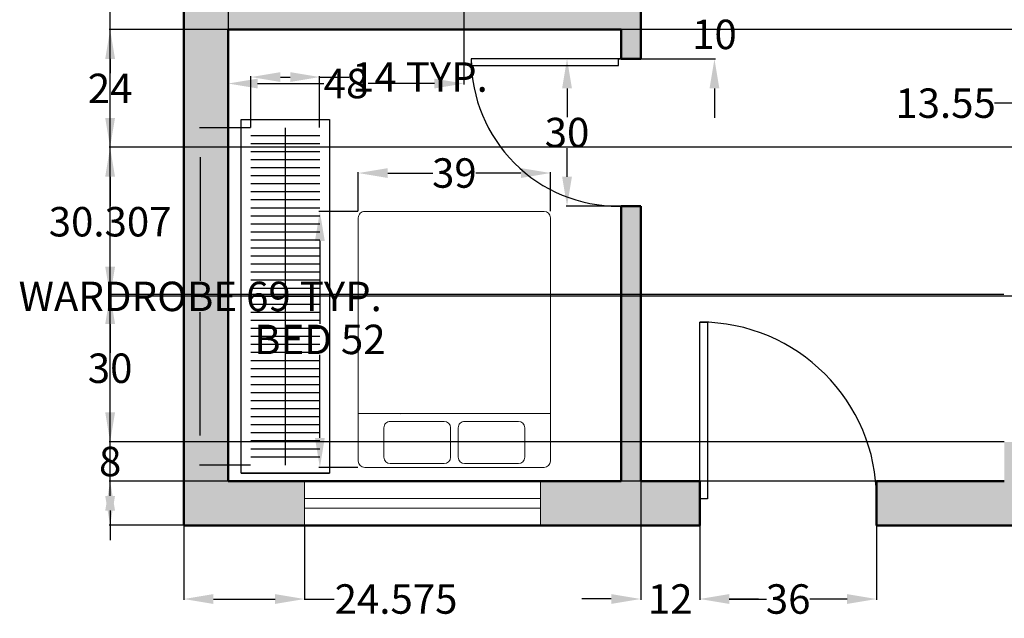
# Model space of a CAD drawing. Units: inches. Extents: x -11 to 341, y -300 to 41.
# Tile 1 of 5: x -9 to 192, y -300 to -178. Entities that reach past the tile are written whole.
import ezdxf

# ---------------------------------------------------------------- set-up
doc = ezdxf.new("R2010")
doc.units = ezdxf.units.IN
doc.header["$MEASUREMENT"] = 0
for name, color, linetype, lineweight in [('A-ANNO-DIMS', 2, 'Continuous', 18), ('A-DOOR', 3, 'Continuous', 25), ('A-FLOR-CASE', 8, 'Continuous', 25), ('A-FURN', 8, 'Continuous', 18), ('A-GLAZ', 4, 'Continuous', 18), ('A-WALL', 7, 'Continuous', 50), ('A-WALL-PATT', 251, 'Continuous', 13)]:
    doc.layers.add(name, color=color, linetype=linetype, lineweight=lineweight)
doc.styles.get("Standard").update_dxf_attribs({"font": 'arial.ttf'})
doc.dimstyles.get("Standard").update_dxf_attribs({"dimtxt": 6, "dimasz": 6, "dimexe": 0.18, "dimexo": 0.0625, "dimgap": 0.09, "dimtad": 0, "dimtih": 1, "dimtoh": 1, "dimdec": 0, "dimzin": 0, "dimdsep": 46, "dimlunit": 4, "dimtxsty": 'Standard', "dimcen": 0.09, "dimadec": 0, "dimazin": 0, "dimtfac": 1, "dimtdec": 0, "dimtofl": 0, "dimtmove": 0, "dimatfit": 3, "dimfxl": 1, "dimtolj": 1, "dimtzin": 0, "dimarcsym": 0})

# ---------------------------------------------------------------- blocks, each defined once
blk = doc.blocks.new('*U13')
for p, q in [((0, 0), (0, 6)), ((40, 0), (40, 6))]:
    blk.add_line(p, q)
blk.add_lwpolyline([(0, 0), (0, -40), (1.75, -40), (1.75, 0)], close=True)
blk.add_arc((0, 0), 40, 270, 0)
blk = doc.blocks.new('*U12')
for p, q in [((0, 0), (0, -6)), ((40, 0), (40, -6))]:
    blk.add_line(p, q)
blk.add_lwpolyline([(0, 0), (0, 40), (1.75, 40), (1.75, 0)], close=True)
blk.add_arc((0, 0), 40, 0, 90)
blk = doc.blocks.new('Bed - Queen')
for p, q in [((2, 0), (57.99999, 0)), ((0, -78.00003), (0, -2)), ((9.99999, -1.2), (26.79998, -1.2)), ((33.19999, -1.2), (49.99999, -1.2)), ((59.99999, -2), (59.99999, -78.00003)), ((7.99999, -12.4), (7.99999, -3.2)), ((28.79998, -3.2), (28.79998, -12.4)), ((31.19999, -12.4), (31.19999, -3.2)), ((51.99999, -3.2), (51.99999, -12.4)), ((9.99999, -14.4), (26.79998, -14.4)), ((33.19999, -14.4), (49.99999, -14.4)), ((59.99999, -16.8), (0, -16.8)), ((46.8, -16.4), (46.79936, -16.4)), ((57.99999, -80.00003), (2, -80.00003))]:
    blk.add_line(p, q)
for centre, start, end in [((2, -2), 90, 180), ((57.99999, -2), 0, 90), ((9.99999, -3.2), 90, 180), ((26.79998, -3.2), 0, 90), ((33.19999, -3.2), 90, 180), ((49.99999, -3.2), 0, 90), ((9.99999, -12.4), 180, 270), ((26.79998, -12.4), 270, 0), ((33.19999, -12.4), 180, 270), ((49.99999, -12.4), 270, 0), ((2, -78.00003), 180, 270), ((57.99999, -78.00003), 270, 0)]:
    blk.add_arc(centre, 2, start, end)
blk = doc.blocks.new('WIN-48IN')
for p, q in [((0, 0), (0, 9)), ((48, 9), (48, 0)), ((0, 5.5), (48, 5.5)), ((0, 3.5), (48, 3.5))]:
    blk.add_line(p, q)
blk = doc.blocks.new('WARDROBE-HANGING-RAIL')
for p, q in [((7, 68.73), (7, 0)), ((14, 67.09), (0, 67.09)), ((14, 65.45), (0, 65.45)), ((14, 63.82), (0, 63.82)), ((14, 62.18), (0, 62.18)), ((14, 60.55), (0, 60.55)), ((14, 58.91), (0, 58.91)), ((14, 57.27), (0, 57.27)), ((14, 55.64), (0, 55.64)), ((14, 54), (0, 54)), ((14, 52.36), (0, 52.36)), ((14, 50.73), (0, 50.73)), ((14, 49.09), (0, 49.09)), ((14, 47.45), (0, 47.45)), ((14, 45.82), (0, 45.82)), ((14, 44.18), (0, 44.18)), ((14, 42.55), (0, 42.55)), ((14, 40.91), (0, 40.91)), ((14, 39.27), (0, 39.27)), ((14, 37.64), (0, 37.64)), ((14, 36), (0, 36)), ((14, 34.36), (0, 34.36)), ((14, 32.73), (0, 32.73)), ((14, 31.09), (0, 31.09)), ((14, 29.45), (0, 29.45)), ((14, 27.82), (0, 27.82)), ((14, 26.18), (0, 26.18)), ((14, 24.55), (0, 24.55)), ((14, 22.91), (0, 22.91)), ((14, 21.27), (0, 21.27)), ((14, 19.64), (0, 19.64)), ((14, 18), (0, 18)), ((14, 16.36), (0, 16.36)), ((14, 14.73), (0, 14.73)), ((14, 13.09), (0, 13.09)), ((14, 11.45), (0, 11.45)), ((14, 9.82), (0, 9.82)), ((14, 8.18), (0, 8.18)), ((14, 6.55), (0, 6.55)), ((14, 4.91), (0, 4.91)), ((14, 3.27), (0, 3.27)), ((14, 1.64), (0, 1.64))]:
    blk.add_line(p, q)
blk = doc.blocks.new('*D23')
at = {"layer": 'A-ANNO-DIMS', "color": 0, "lineweight": -2, "transparency": 16777216}
for p, q in [((60.01, -216.66), (52.07, -216.66)), ((52.25, -222.66), (52.25, -239.58)), ((52.25, -262.81), (52.25, -245.89)), ((60.01, -268.81), (52.07, -268.81))]:
    blk.add_line(p, q, dxfattribs=at)
at = {"layer": 'A-ANNO-DIMS', "color": 0, "transparency": 16777216}
for points in [[(51.25, -222.66), (53.25, -222.66), (52.25, -216.66)], [(51.25, -262.81), (53.25, -262.81), (52.25, -268.81)]]:
    blk.add_solid(points, dxfattribs=at)
at = {"layer": 'Defpoints', "color": 0, "transparency": 16777216}
for p in [(60.08, -216.66), (52.25, -268.81), (60.08, -268.81)]:
    blk.add_point(p, dxfattribs=at)
at = {"layer": 'A-ANNO-DIMS', "color": 0, "transparency": 16777216, "insert": (52.25, -242.73), "char_height": 6, "attachment_point": 5}
blk.add_mtext('\\A1;BED 52', dxfattribs=at)
blk = doc.blocks.new('*D24')
at = {"layer": 'A-ANNO-DIMS', "color": 0, "lineweight": -2, "transparency": 16777216}
for p, q in [((60.08, -216.6), (60.08, -208.66)), ((66.08, -208.84), (75.24, -208.84)), ((93.18, -208.84), (84.02, -208.84)), ((99.18, -216.6), (99.18, -208.66))]:
    blk.add_line(p, q, dxfattribs=at)
at = {"layer": 'A-ANNO-DIMS', "color": 0, "transparency": 16777216}
for points in [[(66.08, -207.84), (66.08, -209.84), (60.08, -208.84)], [(93.18, -207.84), (93.18, -209.84), (99.18, -208.84)]]:
    blk.add_solid(points, dxfattribs=at)
at = {"layer": 'Defpoints', "color": 0, "transparency": 16777216}
for p in [(60.08, -208.84), (60.08, -216.66), (99.18, -216.66)]:
    blk.add_point(p, dxfattribs=at)
at = {"layer": 'A-ANNO-DIMS', "color": 0, "transparency": 16777216, "insert": (79.63, -208.84), "char_height": 6, "attachment_point": 5}
blk.add_mtext('\\A1;39', dxfattribs=at)
blk = doc.blocks.new('*D27')
at = {"layer": 'A-ANNO-DIMS', "color": 0, "lineweight": -2, "transparency": 16777216}
for p, q in [((38.15, -199.6), (27.72, -199.6)), ((27.9, -205.6), (27.9, -230.77)), ((27.9, -262.33), (27.9, -237.16)), ((38.15, -268.33), (27.72, -268.33))]:
    blk.add_line(p, q, dxfattribs=at)
at = {"layer": 'A-ANNO-DIMS', "color": 0, "transparency": 16777216}
for points in [[(26.9, -205.6), (28.9, -205.6), (27.9, -199.6)], [(26.9, -262.33), (28.9, -262.33), (27.9, -268.33)]]:
    blk.add_solid(points, dxfattribs=at)
at = {"layer": 'Defpoints', "color": 0, "transparency": 16777216}
for p in [(27.9, -199.6), (38.21, -199.6), (38.21, -268.33)]:
    blk.add_point(p, dxfattribs=at)
at = {"layer": 'A-ANNO-DIMS', "color": 0, "transparency": 16777216, "insert": (27.9, -233.97), "char_height": 6, "attachment_point": 5}
blk.add_mtext('\\A1;WARDROBE 69 TYP.', dxfattribs=at)
blk = doc.blocks.new('*D28')
at = {"layer": 'A-ANNO-DIMS', "color": 0, "lineweight": -2, "transparency": 16777216}
for p, q in [((38.21, -199.54), (38.21, -189.11)), ((44.21, -189.29), (46.21, -189.29)), ((52.21, -199.54), (52.21, -189.11)), ((52.21, -189.29), (58.21, -189.29))]:
    blk.add_line(p, q, dxfattribs=at)
at = {"layer": 'A-ANNO-DIMS', "color": 0, "transparency": 16777216}
for points in [[(44.21, -188.29), (44.21, -190.29), (38.21, -189.29)], [(46.21, -188.29), (46.21, -190.29), (52.21, -189.29)]]:
    blk.add_solid(points, dxfattribs=at)
at = {"layer": 'Defpoints', "color": 0, "transparency": 16777216}
for p in [(52.21, -189.29), (38.21, -199.6), (52.21, -199.6)]:
    blk.add_point(p, dxfattribs=at)
at = {"layer": 'A-ANNO-DIMS', "color": 0, "transparency": 16777216, "insert": (72.62, -189.29), "char_height": 6, "attachment_point": 5}
blk.add_mtext('\\A1;14 TYP.', dxfattribs=at)
blk = doc.blocks.new('*D46')
at = {"layer": 'A-ANNO-DIMS', "color": 0, "lineweight": -2, "transparency": 16777216}
for p, q in [((24.5, 19.4), (9.38, 19.4)), ((9.56, 13.4), (9.56, -127.45)), ((9.56, -274.6), (9.56, -133.76)), ((24.5, -280.6), (9.38, -280.6))]:
    blk.add_line(p, q, dxfattribs=at)
at = {"layer": 'A-ANNO-DIMS', "color": 0, "transparency": 16777216}
for points in [[(8.56, 13.4), (10.56, 13.4), (9.56, 19.4)], [(8.56, -274.6), (10.56, -274.6), (9.56, -280.6)]]:
    blk.add_solid(points, dxfattribs=at)
at = {"layer": 'Defpoints', "color": 0, "transparency": 16777216}
for p in [(9.56, 19.4), (24.57, 19.4), (24.57, -280.6)]:
    blk.add_point(p, dxfattribs=at)
at = {"layer": 'A-ANNO-DIMS', "color": 0, "transparency": 16777216, "insert": (9.56, -130.6), "char_height": 6, "attachment_point": 5}
blk.add_mtext('\\A1;300', dxfattribs=at)
blk = doc.blocks.new('*D50')
at = {"layer": 'A-ANNO-DIMS', "color": 0, "lineweight": -2, "transparency": 16777216}
for p, q in [((24.57, -280.67), (24.57, -295.79)), ((49.14, -280.67), (49.14, -295.79)), ((30.57, -295.61), (43.14, -295.61)), ((49.14, -295.61), (55.14, -295.61))]:
    blk.add_line(p, q, dxfattribs=at)
at = {"layer": 'A-ANNO-DIMS', "color": 0, "transparency": 16777216}
for points in [[(30.57, -294.61), (30.57, -296.61), (24.57, -295.61)], [(43.14, -294.61), (43.14, -296.61), (49.14, -295.61)]]:
    blk.add_solid(points, dxfattribs=at)
at = {"layer": 'Defpoints', "color": 0, "transparency": 16777216}
for p in [(24.57, -280.6), (49.14, -280.6), (49.14, -295.61)]:
    blk.add_point(p, dxfattribs=at)
at = {"layer": 'A-ANNO-DIMS', "color": 0, "transparency": 16777216, "insert": (67.76, -295.61), "char_height": 6, "attachment_point": 5}
blk.add_mtext('\\A1;24.575', dxfattribs=at)
blk = doc.blocks.new('*D51')
at = {"layer": 'A-ANNO-DIMS', "color": 0, "lineweight": -2, "transparency": 16777216}
for p, q in [((117.565121, -271.665765), (117.565121, -295.785265)), ((129.565121, -271.665765), (129.565121, -295.785265)), ((111.565121, -295.605265), (105.565121, -295.605265)), ((135.565121, -295.605265), (141.565121, -295.605265))]:
    blk.add_line(p, q, dxfattribs=at)
at = {"layer": 'A-ANNO-DIMS', "color": 0, "transparency": 16777216}
for points in [[(111.565121, -294.605265), (111.565121, -296.605265), (117.565121, -295.605265)], [(135.565121, -294.605265), (135.565121, -296.605265), (129.565121, -295.605265)]]:
    blk.add_solid(points, dxfattribs=at)
at = {"layer": 'Defpoints', "color": 0, "transparency": 16777216}
for p in [(117.565121, -271.603265), (129.565121, -271.603265), (129.565121, -295.605265)]:
    blk.add_point(p, dxfattribs=at)
at = {"layer": 'A-ANNO-DIMS', "color": 0, "transparency": 16777216, "insert": (123.565121, -295.605265), "char_height": 6, "attachment_point": 5}
blk.add_mtext('\\A1;12', dxfattribs=at)
blk = doc.blocks.new('*D52')
at = {"layer": 'A-ANNO-DIMS', "color": 0, "lineweight": -2, "transparency": 16777216}
for p, q in [((129.57, -280.67), (129.57, -295.79)), ((165.57, -280.67), (165.57, -295.79)), ((135.57, -295.61), (143.18, -295.61)), ((159.57, -295.61), (151.95, -295.61))]:
    blk.add_line(p, q, dxfattribs=at)
at = {"layer": 'A-ANNO-DIMS', "color": 0, "transparency": 16777216}
for points in [[(135.57, -294.61), (135.57, -296.61), (129.57, -295.61)], [(159.57, -294.61), (159.57, -296.61), (165.57, -295.61)]]:
    blk.add_solid(points, dxfattribs=at)
at = {"layer": 'Defpoints', "color": 0, "transparency": 16777216}
for p in [(129.57, -280.6), (165.57, -280.6), (165.57, -295.61)]:
    blk.add_point(p, dxfattribs=at)
at = {"layer": 'A-ANNO-DIMS', "color": 0, "transparency": 16777216, "insert": (147.57, -295.61), "char_height": 6, "attachment_point": 5}
blk.add_mtext('\\A1;36', dxfattribs=at)
blk = doc.blocks.new('*D61')
at = {"layer": 'A-ANNO-DIMS', "color": 0, "lineweight": -2, "transparency": 16777216}
for p, q in [((33.57, -175.67), (33.57, -190.79)), ((81.57, -175.67), (81.57, -190.79)), ((39.57, -190.61), (53.05, -190.61)), ((75.57, -190.61), (62.08, -190.61))]:
    blk.add_line(p, q, dxfattribs=at)
at = {"layer": 'A-ANNO-DIMS', "color": 0, "transparency": 16777216}
for points in [[(39.57, -189.61), (39.57, -191.61), (33.57, -190.61)], [(75.57, -189.61), (75.57, -191.61), (81.57, -190.61)]]:
    blk.add_solid(points, dxfattribs=at)
at = {"layer": 'Defpoints', "color": 0, "transparency": 16777216}
for p in [(33.57, -175.6), (81.57, -175.6), (33.57, -190.61)]:
    blk.add_point(p, dxfattribs=at)
at = {"layer": 'A-ANNO-DIMS', "color": 0, "transparency": 16777216, "insert": (57.57, -190.61), "char_height": 6, "attachment_point": 5}
blk.add_mtext('\\A1;48', dxfattribs=at)
blk = doc.blocks.new('*D70')
at = {"layer": 'A-ANNO-DIMS', "color": 0, "lineweight": -2, "transparency": 16777216}
for p, q in [((132.567121, -169.603265), (132.567121, -163.603265)), ((117.627621, -175.603265), (132.747121, -175.603265)), ((117.627621, -185.603265), (132.747121, -185.603265)), ((132.567121, -191.603265), (132.567121, -197.603265))]:
    blk.add_line(p, q, dxfattribs=at)
at = {"layer": 'A-ANNO-DIMS', "color": 0, "transparency": 16777216}
for points in [[(131.567121, -169.603265), (133.567121, -169.603265), (132.567121, -175.603265)], [(131.567121, -191.603265), (133.567121, -191.603265), (132.567121, -185.603265)]]:
    blk.add_solid(points, dxfattribs=at)
at = {"layer": 'Defpoints', "color": 0, "transparency": 16777216}
for p in [(117.565121, -175.603265), (117.565121, -185.603265), (132.567121, -185.603265)]:
    blk.add_point(p, dxfattribs=at)
at = {"layer": 'A-ANNO-DIMS', "color": 0, "transparency": 16777216, "insert": (132.567121, -180.603265), "char_height": 6, "attachment_point": 5}
blk.add_mtext('\\A1;10', dxfattribs=at)
blk = doc.blocks.new('*D71')
at = {"layer": 'A-ANNO-DIMS', "color": 0, "lineweight": -2, "transparency": 16777216}
for p, q in [((117.5, -185.6), (102.38, -185.6)), ((102.56, -191.6), (102.56, -197.45)), ((102.56, -209.6), (102.56, -203.76)), ((117.5, -215.6), (102.38, -215.6))]:
    blk.add_line(p, q, dxfattribs=at)
at = {"layer": 'A-ANNO-DIMS', "color": 0, "transparency": 16777216}
for points in [[(101.56, -191.6), (103.56, -191.6), (102.56, -185.6)], [(101.56, -209.6), (103.56, -209.6), (102.56, -215.6)]]:
    blk.add_solid(points, dxfattribs=at)
at = {"layer": 'Defpoints', "color": 0, "transparency": 16777216}
for p in [(102.56, -185.6), (117.57, -185.6), (117.57, -215.6)]:
    blk.add_point(p, dxfattribs=at)
at = {"layer": 'A-ANNO-DIMS', "color": 0, "transparency": 16777216, "insert": (102.56, -200.6), "char_height": 6, "attachment_point": 5}
blk.add_mtext('\\A1;30', dxfattribs=at)
blk = doc.blocks.new('*D72')
at = {"layer": 'A-ANNO-DIMS', "color": 0, "lineweight": -2, "transparency": 16777216}
for p, q in [((9.563121, -257.603265), (9.563121, -251.603265)), ((191.502621, -263.603265), (9.383121, -263.603265)), ((191.502621, -271.603265), (9.383121, -271.603265)), ((9.563121, -277.603265), (9.563121, -283.603265))]:
    blk.add_line(p, q, dxfattribs=at)
at = {"layer": 'A-ANNO-DIMS', "color": 0, "transparency": 16777216}
for points in [[(8.563121, -257.603265), (10.563121, -257.603265), (9.563121, -263.603265)], [(8.563121, -277.603265), (10.563121, -277.603265), (9.563121, -271.603265)]]:
    blk.add_solid(points, dxfattribs=at)
at = {"layer": 'Defpoints', "color": 0, "transparency": 16777216}
for p in [(191.565121, -263.603265), (9.563121, -271.603265), (191.565121, -271.603265)]:
    blk.add_point(p, dxfattribs=at)
at = {"layer": 'A-ANNO-DIMS', "color": 0, "transparency": 16777216, "insert": (9.563121, -267.603265), "char_height": 6, "attachment_point": 5}
blk.add_mtext('\\A1;8', dxfattribs=at)
blk = doc.blocks.new('*D73')
at = {"layer": 'A-ANNO-DIMS', "color": 0, "lineweight": -2, "transparency": 16777216}
for p, q in [((191.5, -233.6), (9.38, -233.6)), ((9.56, -239.6), (9.56, -245.45)), ((9.56, -257.6), (9.56, -251.76)), ((191.5, -263.6), (9.38, -263.6))]:
    blk.add_line(p, q, dxfattribs=at)
at = {"layer": 'A-ANNO-DIMS', "color": 0, "transparency": 16777216}
for points in [[(8.56, -239.6), (10.56, -239.6), (9.56, -233.6)], [(8.56, -257.6), (10.56, -257.6), (9.56, -263.6)]]:
    blk.add_solid(points, dxfattribs=at)
at = {"layer": 'Defpoints', "color": 0, "transparency": 16777216}
for p in [(9.56, -233.6), (191.57, -233.6), (191.57, -263.6)]:
    blk.add_point(p, dxfattribs=at)
at = {"layer": 'A-ANNO-DIMS', "color": 0, "transparency": 16777216, "insert": (9.56, -248.6), "char_height": 6, "attachment_point": 5}
blk.add_mtext('\\A1;30', dxfattribs=at)
blk = doc.blocks.new('*D74')
at = {"layer": 'A-ANNO-DIMS', "color": 0, "lineweight": -2, "transparency": 16777216}
for p, q in [((209.05, -179.6), (9.38, -179.6)), ((9.56, -185.6), (9.56, -188.5)), ((9.56, -197.6), (9.56, -194.71)), ((209.05, -203.6), (9.38, -203.6))]:
    blk.add_line(p, q, dxfattribs=at)
at = {"layer": 'A-ANNO-DIMS', "color": 0, "transparency": 16777216}
for points in [[(8.56, -185.6), (10.56, -185.6), (9.56, -179.6)], [(8.56, -197.6), (10.56, -197.6), (9.56, -203.6)]]:
    blk.add_solid(points, dxfattribs=at)
at = {"layer": 'Defpoints', "color": 0, "transparency": 16777216}
for p in [(209.11, -179.6), (9.56, -203.6), (209.11, -203.6)]:
    blk.add_point(p, dxfattribs=at)
at = {"layer": 'A-ANNO-DIMS', "color": 0, "transparency": 16777216, "insert": (9.56, -191.6), "char_height": 6, "attachment_point": 5}
blk.add_mtext('\\A1;24', dxfattribs=at)
blk = doc.blocks.new('*D75')
at = {"layer": 'A-ANNO-DIMS', "color": 0, "lineweight": -2, "transparency": 16777216}
for p, q in [((195.57, -179.67), (195.57, -194.79)), ((209.11, -179.67), (209.11, -194.79)), ((195.57, -194.61), (189.57, -194.61)), ((203.11, -194.61), (201.57, -194.61))]:
    blk.add_line(p, q, dxfattribs=at)
at = {"layer": 'A-ANNO-DIMS', "color": 0, "transparency": 16777216}
for points in [[(201.57, -193.61), (201.57, -195.61), (195.57, -194.61)], [(203.11, -193.61), (203.11, -195.61), (209.11, -194.61)]]:
    blk.add_solid(points, dxfattribs=at)
at = {"layer": 'Defpoints', "color": 0, "transparency": 16777216}
for p in [(195.57, -179.6), (209.11, -179.6), (195.57, -194.61)]:
    blk.add_point(p, dxfattribs=at)
at = {"layer": 'A-ANNO-DIMS', "color": 0, "transparency": 16777216, "insert": (179.61, -194.61), "char_height": 6, "attachment_point": 5}
blk.add_mtext('\\A1;13.55', dxfattribs=at)
blk = doc.blocks.new('*D76')
at = {"layer": 'A-ANNO-DIMS', "color": 0, "lineweight": -2, "transparency": 16777216}
for p, q in [((255.5, -203.6), (9.38, -203.6)), ((9.56, -209.6), (9.56, -215.6)), ((9.56, -227.91), (9.56, -221.91)), ((255.5, -233.91), (9.38, -233.91))]:
    blk.add_line(p, q, dxfattribs=at)
at = {"layer": 'A-ANNO-DIMS', "color": 0, "transparency": 16777216}
for points in [[(8.56, -209.6), (10.56, -209.6), (9.56, -203.6)], [(8.56, -227.91), (10.56, -227.91), (9.56, -233.91)]]:
    blk.add_solid(points, dxfattribs=at)
at = {"layer": 'Defpoints', "color": 0, "transparency": 16777216}
for p in [(9.56, -203.6), (255.57, -203.6), (255.57, -233.91)]:
    blk.add_point(p, dxfattribs=at)
at = {"layer": 'A-ANNO-DIMS', "color": 0, "transparency": 16777216, "insert": (9.56, -218.76), "char_height": 6, "attachment_point": 5}
blk.add_mtext('\\A1;30.307', dxfattribs=at)

msp = doc.modelspace()

# ---------------------------------------------------------------- hatches: boundary and pattern name
at = {"layer": 'A-WALL-PATT'}
h = msp.add_hatch(color=256, dxfattribs=at)
h.dxf.hatch_style = 1
h.paths.add_polyline_path([(24.5651, -280.6033), (49.1398, -280.6033), (49.1398, -271.6033), (33.5651, -271.6033), (33.5651, -179.6033), (113.5651, -179.6033), (113.5651, -185.6033), (117.5651, -185.6033), (117.5651, -175.6033), (85.5651, -175.6033), (85.5651, -127.6033), (81.5651, -127.6033), (81.5651, -175.6033), (33.5651, -175.6033), (33.5651, -138.096), (24.5651, -138.096)])
h = msp.add_hatch(color=256, dxfattribs=at)
h.dxf.hatch_style = 1
h.paths.add_polyline_path([(129.5651, -271.6033), (117.5651, -271.6033), (117.5651, -215.6033), (113.5651, -215.6033), (113.5651, -271.6033), (97.1398, -271.6033), (97.1398, -280.6033), (129.5651, -280.6033), (129.5651, -275.2033)])
h = msp.add_hatch(color=256, dxfattribs=at)
h.dxf.hatch_style = 1
h.paths.add_polyline_path([(215.5868, -280.6033), (215.5868, -271.6033), (195.5651, -271.6033), (195.5651, -263.6033), (191.5651, -263.6033), (191.5651, -271.6033), (165.5651, -271.6033), (165.5651, -280.6033)])

# ---------------------------------------------------------------- linework, layer by layer
at = {"layer": 'A-FLOR-CASE'}
msp.add_lwpolyline([(36.2111, -269.9669), (36.2111, -197.9669), (54.2111, -197.9669), (54.2111, -269.9669), (36.2111, -269.9669), (54.2111, -269.9669)], dxfattribs=at)
at = {"layer": 'A-WALL'}
for p, q in [((117.5651, -185.6033), (117.5651, -175.6033)), ((33.5651, -271.6033), (33.5651, -179.6033)), ((113.5651, -179.6033), (33.5651, -179.6033)), ((113.5651, -185.6033), (113.5651, -179.6033)), ((113.5651, -185.6033), (117.5651, -185.6033)), ((113.5651, -271.6033), (113.5651, -215.6033)), ((113.5651, -215.6033), (117.5651, -215.6033)), ((117.5651, -271.6033), (117.5651, -215.6033)), ((113.5651, -271.6033), (33.5651, -271.6033)), ((129.5651, -271.6033), (117.5651, -271.6033)), ((129.5651, -271.6033), (129.5651, -280.6033)), ((191.5651, -271.6033), (165.5651, -271.6033)), ((165.5651, -271.6033), (165.5651, -280.6033))]:
    msp.add_line(p, q, dxfattribs=at)
msp.add_lwpolyline([(129.5651, -280.6033), (24.5651, -280.6033), (24.5651, 19.3967), (288.5651, 19.3967), (288.5651, -280.6033), (165.5651, -280.6033)], dxfattribs=at)

# ---------------------------------------------------------------- block references
at = {"layer": 'A-DOOR', "xscale": 0.75, "yscale": 0.75, "zscale": 0.75, "rotation": 270}
msp.add_blockref('*U13', (113.0651, -185.6033), dxfattribs=at)
at = {"layer": 'A-DOOR', "xscale": 0.9, "yscale": 0.9, "zscale": 0.9}
msp.add_blockref('*U12', (129.5651, -275.2033), dxfattribs=at)
at = {"layer": 'A-FLOR-CASE'}
msp.add_blockref('WARDROBE-HANGING-RAIL', (38.2115, -268.3304), dxfattribs=at)
at = {"layer": 'A-FURN', "xscale": 0.6518282349868454, "yscale": 0.6518282349868454, "zscale": 0.6518282349868454, "rotation": 180}
msp.add_blockref('Bed - Queen', (99.1848, -268.8057), dxfattribs=at)
at = {"layer": 'A-GLAZ'}
msp.add_blockref('WIN-48IN', (49.1397, -280.603), dxfattribs=at)

# ---------------------------------------------------------------- dimensions: what is measured, and where the dimension line sits
at = {"layer": 'A-ANNO-DIMS'}
for base, p1, p2, angle, override, picture, middle in [((9.5631, 19.3967), (24.5651, -280.6033), (24.5651, 19.3967), 90, {"dimdec": 0, "dimlfac": 1, "dimrnd": 0, "dimzin": 0, "dimdsep": 46, "dimlunit": 2}, '*D46', (9.5631, -130.6033)), ((132.5671, -185.6033), (117.5651, -175.6033), (117.5651, -185.6033), 270, {"dimdec": 0, "dimlfac": 1, "dimrnd": 0, "dimzin": 0, "dimdsep": 46, "dimlunit": 2}, '*D70', (132.5671, -180.6033)), ((33.5651, -190.6053), (81.5651, -175.6033), (33.5651, -175.6033), 180, {"dimdec": 0, "dimlfac": 1, "dimrnd": 0, "dimzin": 0, "dimdsep": 46, "dimlunit": 2}, '*D61', (57.5651, -190.6053)), ((9.5631, -203.6033), (209.1143, -179.6033), (209.1143, -203.6033), 90, {"dimdec": 0, "dimlfac": 1, "dimrnd": 0, "dimzin": 0, "dimdsep": 46, "dimlunit": 2}, '*D74', (9.5631, -191.6033)), ((195.5651, -194.6053), (209.1143, -179.6033), (195.5651, -179.6033), 180, {"dimdec": 2, "dimlfac": 1, "dimrnd": 0, "dimzin": 0, "dimdsep": 46, "dimlunit": 2}, '*D75', (179.6115, -194.6053)), ((102.5631, -185.6033), (117.5651, -215.6033), (117.5651, -185.6033), 90, {"dimdec": 0, "dimlfac": 1, "dimrnd": 0, "dimzin": 0, "dimdsep": 46, "dimlunit": 2}, '*D71', (102.5631, -200.6033)), ((9.5631, -203.6033), (255.5651, -233.9102), (255.5651, -203.6033), 90, {"dimdec": 3, "dimlfac": 1, "dimrnd": 0, "dimzin": 0, "dimdsep": 46, "dimlunit": 2}, '*D76', (9.5631, -218.7567)), ((60.0751, -208.8375), (99.1848, -216.6594), (60.0751, -216.6594), 180, {"dimdec": 0, "dimlfac": 1, "dimrnd": 0, "dimzin": 0, "dimdsep": 46, "dimlunit": 2}, '*D24', (79.63, -208.8375)), ((9.5631, -233.6033), (191.5651, -263.6033), (191.5651, -233.6033), 90, {"dimdec": 0, "dimlfac": 1, "dimrnd": 0, "dimzin": 0, "dimdsep": 46, "dimlunit": 2}, '*D73', (9.5631, -248.6033)), ((9.5631, -271.6033), (191.5651, -263.6033), (191.5651, -271.6033), 90, {"dimdec": 0, "dimlfac": 1, "dimrnd": 0, "dimzin": 0, "dimdsep": 46, "dimlunit": 2}, '*D72', (9.5631, -267.6033))]:
    dim = msp.add_linear_dim(base=base, p1=p1, p2=p2, angle=angle, dimstyle='Standard', override=override, dxfattribs=at)
    dim.commit()
    dim.dimension.update_dxf_attribs({"geometry": picture, "text_midpoint": middle})
dim = msp.add_linear_dim(base=(52.2111, -189.2942), p1=(38.2111, -199.6033), p2=(52.2111, -199.6033), text='<> TYP.', dimstyle='Standard', override={"dimdec": 0, "dimlfac": 1, "dimrnd": 0, "dimzin": 0, "dimdsep": 46, "dimlunit": 2}, dxfattribs=at)
dim.commit()
dim.dimension.update_dxf_attribs({"geometry": '*D28', "text_midpoint": (72.6217, -189.2942)})
for base, p1, p2, angle, text, picture, middle in [((27.902, -199.6033), (38.2111, -268.3305), (38.2111, -199.6033), 90, 'WARDROBE <> TYP.', '*D27', (27.902, -233.9669)), ((52.2532, -268.8057), (60.0751, -216.6594), (60.0751, -268.8057), 270, 'BED <>', '*D23', (52.2532, -242.7326))]:
    dim = msp.add_linear_dim(base=base, p1=p1, p2=p2, angle=angle, text=text, dimstyle='Standard', override={"dimdec": 0, "dimlfac": 1, "dimrnd": 0, "dimzin": 0, "dimdsep": 46, "dimlunit": 2}, dxfattribs=at)
    dim.commit()
    dim.dimension.update_dxf_attribs({"geometry": picture, "text_midpoint": middle})
for base, p1, p2, override, picture, middle in [((129.5651, -295.6053), (117.5651, -271.6033), (129.5651, -271.6033), {"dimdec": 0, "dimlfac": 1, "dimrnd": 0, "dimzin": 0, "dimdsep": 46, "dimlunit": 2}, '*D51', (123.5651, -295.6053)), ((49.1398, -295.6053), (24.5651, -280.6033), (49.1398, -280.6033), {"dimdec": 3, "dimlfac": 1, "dimrnd": 0, "dimzin": 0, "dimdsep": 46, "dimlunit": 2}, '*D50', (67.7578, -295.6053)), ((165.5651, -295.6053), (129.5651, -280.6033), (165.5651, -280.6033), {"dimdec": 0, "dimlfac": 1, "dimrnd": 0, "dimzin": 0, "dimdsep": 46, "dimlunit": 2}, '*D52', (147.5651, -295.6053))]:
    dim = msp.add_linear_dim(base=base, p1=p1, p2=p2, dimstyle='Standard', override=override, dxfattribs=at)
    dim.commit()
    dim.dimension.update_dxf_attribs({"geometry": picture, "text_midpoint": middle})

doc.saveas('drawing.dxf')
